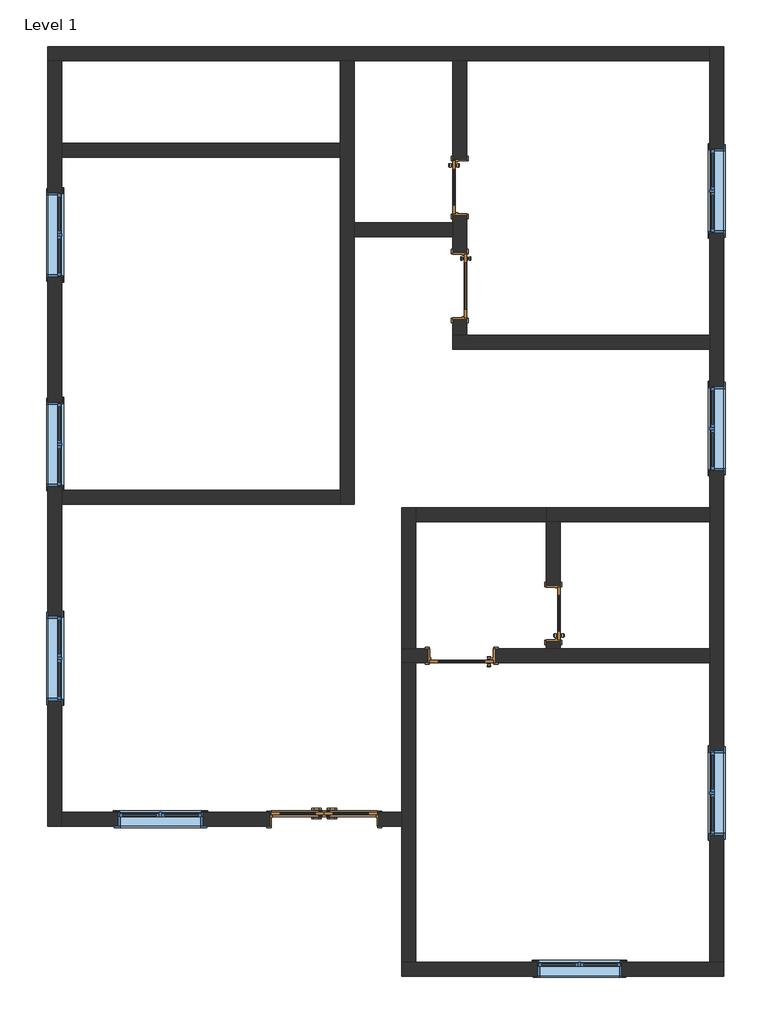
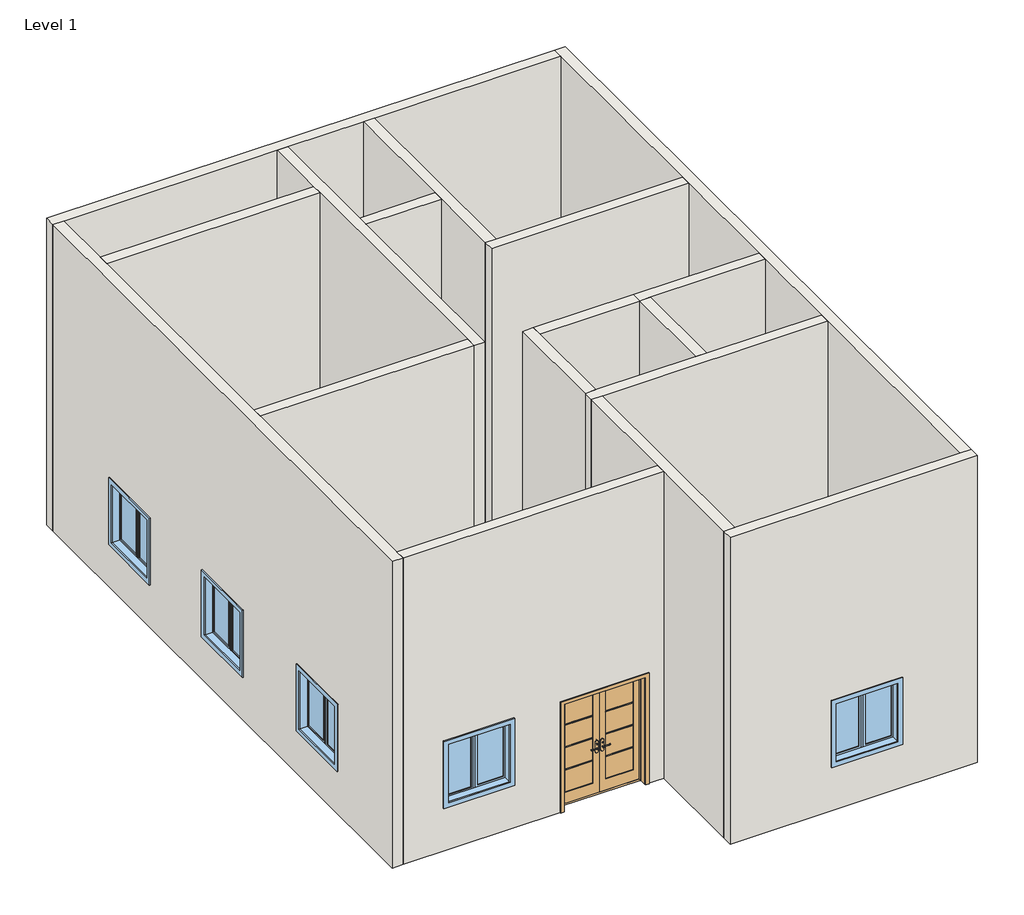
# One storey: 17 walls, 8 windows, 5 doors.
"""IFC4 building model written with IfcOpenShell, lengths in millimetres."""

from ifc_helpers import new_model, si_unit, frame, origin, origin_with_axes, place, context, project, spatial, polyline, outline, extrude, faceted_brep, transform, mapped, element, save
from components import door_34824ff4, door_975671f7, door_b5100634, window_0862ab64

model = new_model("IFC4")

# Units and contexts
model_context = context("Model", 3, world=origin())
ifc_project = project(units=[si_unit("LENGTHUNIT", "METRE", prefix="MILLI")], contexts=[model_context])

# Site, building, storey
site = spatial("IfcSite", under=ifc_project)
building = spatial("IfcBuilding", under=site)
storey = spatial("IfcBuildingStorey", under=building, Name="Level 1", Elevation=0.0)

# Doors
placement = place(None, origin())
door_shape = door_34824ff4(model_context)
element("IfcDoor", 1, ObjectType="Door-Exterior-Double-Full Glass-Wood_Clad : 60\" x 84\"", at=placement, inside=storey, context=model_context, shape_type="MappedRepresentation", body=[
    mapped(door_shape, transform((20054.3621321, 6414.9686058, 0.0), x_axis=(1.0, 0.0, 0.0), y_axis=(0.0, 1.0, 0.0), z_axis=(0.0, 0.0, 1.0))),
])
door_2_shape = door_975671f7(model_context)
element("IfcDoor", 2, ObjectType="Door-Interior-Single-1_Panel-Wood : 30\" x 80\"", at=placement, inside=storey, context=model_context, shape_type="MappedRepresentation", body=[
    mapped(door_2_shape, transform((22006.9871321, 15530.3936058, 0.0), x_axis=(0.0, -1.0, 0.0), y_axis=(1.0, 0.0, 0.0), z_axis=(0.0, 0.0, 1.0))),
])
element("IfcDoor", 3, ObjectType="Door-Interior-Single-1_Panel-Wood : 30\" x 80\"", at=placement, inside=storey, context=model_context, shape_type="MappedRepresentation", body=[
    mapped(door_2_shape, transform((23359.5371321, 9383.5936058, 0.0), x_axis=(0.0, 1.0, 0.0), y_axis=(-1.0, 0.0, 0.0), z_axis=(0.0, 0.0, 1.0))),
])
door_3_shape = door_b5100634(model_context)
element("IfcDoor", 4, ObjectType="Door-Interior-Single-3_Panel_Vert-Wood : 36\" x 80\"", at=placement, inside=storey, context=model_context, shape_type="MappedRepresentation", body=[
    mapped(door_3_shape, transform((22013.3371321, 14107.9936058, 0.0), x_axis=(0.0, -1.0, 0.0), y_axis=(1.0, 0.0, 0.0), z_axis=(0.0, 0.0, 1.0))),
])
element("IfcDoor", 5, ObjectType="Door-Interior-Single-3_Panel_Vert-Wood : 36\" x 80\"", at=placement, inside=storey, context=model_context, shape_type="MappedRepresentation", body=[
    mapped(door_3_shape, transform((22035.5621321, 8770.8186058, 0.0), x_axis=(-1.0, 0.0, 0.0), y_axis=(0.0, -1.0, 0.0), z_axis=(0.0, 0.0, 1.0))),
])

# Walls
element("IfcWall", 6, ObjectType="Generic - 8\"", at=placement, inside=storey, context=model_context, shape_type="Brep", body=[
    faceted_brep([(16066.5621321, 17359.1936058, 0.0), (16269.7621321, 17359.1936058, 0.0), (20282.9621321, 17359.1936058, 0.0), (20486.1621321, 17359.1936058, 0.0), (21908.5621321, 17359.1936058, 0.0), (22111.7621321, 17359.1936058, 0.0), (25616.9621321, 17359.1936058, 0.0), (25616.9621321, 17359.1936058, 6096.0), (22111.7621321, 17359.1936058, 6096.0), (21908.5621321, 17359.1936058, 6096.0), (20486.1621321, 17359.1936058, 6096.0), (20282.9621321, 17359.1936058, 6096.0), (16269.7621321, 17359.1936058, 6096.0), (16066.5621321, 17359.1936058, 6096.0), (16066.5621321, 17562.3936058, 0.0), (16066.5621321, 17562.3936058, 6096.0), (25616.9621321, 17562.3936058, 6096.0), (25616.9621321, 17562.3936058, 0.0)], [[[0, 1, 2, 3, 4, 5, 6, 7, 8, 9, 10, 11, 12, 13]], [[14, 15, 16, 17]], [[6, 5, 4, 3, 2, 1, 0, 14, 17]], [[13, 12, 11, 10, 9, 8, 7, 16, 15]], [[0, 13, 15, 14]], [[7, 6, 17, 16]]]),
])
element("IfcWall", 7, ObjectType="Generic - 8\"", at=placement, inside=storey, context=model_context, shape_type="Brep", body=[
    faceted_brep([(16269.7621321, 6310.1936058, 0.0), (16269.7621321, 6513.3936058, 0.0), (16269.7621321, 10958.3936058, 0.0), (16269.7621321, 11161.5936058, 0.0), (16269.7621321, 15962.1936058, 0.0), (16269.7621321, 16165.3936058, 0.0), (16269.7621321, 17359.1936058, 0.0), (16269.7621321, 17359.1936058, 6096.0), (16269.7621321, 16165.3936058, 6096.0), (16269.7621321, 15962.1936058, 6096.0), (16269.7621321, 11161.5936058, 6096.0), (16269.7621321, 10958.3936058, 6096.0), (16269.7621321, 6513.3936058, 6096.0), (16269.7621321, 6310.1936058, 6096.0), (16269.7621321, 8126.2936058, 2133.6), (16269.7621321, 9345.4936058, 2133.6), (16269.7621321, 9345.4936058, 914.4), (16269.7621321, 8126.2936058, 914.4), (16269.7621321, 11212.3936058, 2133.6), (16269.7621321, 12431.5936058, 2133.6), (16269.7621321, 12431.5936058, 914.4), (16269.7621321, 11212.3936058, 914.4), (16269.7621321, 14234.9936058, 2133.6), (16269.7621321, 15454.1936058, 2133.6), (16269.7621321, 15454.1936058, 914.4), (16269.7621321, 14234.9936058, 914.4), (16066.5621321, 6310.1936058, 0.0), (16066.5621321, 6310.1936058, 6096.0), (16066.5621321, 17359.1936058, 6096.0), (16066.5621321, 17359.1936058, 0.0), (16066.5621321, 8126.2936058, 2133.6), (16066.5621321, 8126.2936058, 914.4), (16066.5621321, 9345.4936058, 914.4), (16066.5621321, 9345.4936058, 2133.6), (16066.5621321, 11212.3936058, 2133.6), (16066.5621321, 11212.3936058, 914.4), (16066.5621321, 12431.5936058, 914.4), (16066.5621321, 12431.5936058, 2133.6), (16066.5621321, 14234.9936058, 2133.6), (16066.5621321, 14234.9936058, 914.4), (16066.5621321, 15454.1936058, 914.4), (16066.5621321, 15454.1936058, 2133.6)], [[[0, 1, 2, 3, 4, 5, 6, 7, 8, 9, 10, 11, 12, 13], [14, 15, 16, 17], [18, 19, 20, 21], [22, 23, 24, 25]], [[26, 27, 28, 29], [30, 31, 32, 33], [34, 35, 36, 37], [38, 39, 40, 41]], [[6, 5, 4, 3, 2, 1, 0, 26, 29]], [[13, 12, 11, 10, 9, 8, 7, 28, 27]], [[7, 6, 29, 28]], [[0, 13, 27, 26]], [[31, 30, 14, 17]], [[32, 31, 17, 16]], [[33, 32, 16, 15]], [[30, 33, 15, 14]], [[35, 34, 18, 21]], [[36, 35, 21, 20]], [[37, 36, 20, 19]], [[34, 37, 19, 18]], [[39, 38, 22, 25]], [[40, 39, 25, 24]], [[41, 40, 24, 23]], [[38, 41, 23, 22]]]),
])
element("IfcWall", 8, ObjectType="Generic - 8\"", at=placement, inside=storey, context=model_context, shape_type="Brep", body=[
    faceted_brep([(25820.1621321, 4354.3936058, 0.0), (25616.9621321, 4354.3936058, 0.0), (21375.1621321, 4354.3936058, 0.0), (21171.9621321, 4354.3936058, 0.0), (21171.9621321, 4354.3936058, 6096.0), (21375.1621321, 4354.3936058, 6096.0), (25616.9621321, 4354.3936058, 6096.0), (25820.1621321, 4354.3936058, 6096.0), (24346.9621321, 4354.3936058, 2133.6), (23127.7621321, 4354.3936058, 2133.6), (23127.7621321, 4354.3936058, 914.4), (24346.9621321, 4354.3936058, 914.4), (25820.1621321, 4151.1936058, 0.0), (25820.1621321, 4151.1936058, 6096.0), (21171.9621321, 4151.1936058, 6096.0), (21171.9621321, 4151.1936058, 0.0), (24346.9621321, 4151.1936058, 2133.6), (24346.9621321, 4151.1936058, 914.4), (23127.7621321, 4151.1936058, 914.4), (23127.7621321, 4151.1936058, 2133.6)], [[[0, 1, 2, 3, 4, 5, 6, 7], [8, 9, 10, 11]], [[12, 13, 14, 15], [16, 17, 18, 19]], [[3, 2, 1, 0, 12, 15]], [[7, 6, 5, 4, 14, 13]], [[0, 7, 13, 12]], [[4, 3, 15, 14]], [[17, 16, 8, 11]], [[18, 17, 11, 10]], [[19, 18, 10, 9]], [[16, 19, 9, 8]]]),
])
element("IfcWall", 9, ObjectType="Generic - 8\"", at=placement, inside=storey, context=model_context, shape_type="Brep", body=[
    faceted_brep([(25616.9621321, 17562.3936058, 0.0), (25616.9621321, 17359.1936058, 0.0), (25616.9621321, 13396.7936058, 0.0), (25616.9621321, 13193.5936058, 0.0), (25616.9621321, 10907.5936058, 0.0), (25616.9621321, 10704.3936058, 0.0), (25616.9621321, 8875.5936058, 0.0), (25616.9621321, 8672.3936058, 0.0), (25616.9621321, 4354.3936058, 0.0), (25616.9621321, 4354.3936058, 6096.0), (25616.9621321, 8672.3936058, 6096.0), (25616.9621321, 8875.5936058, 6096.0), (25616.9621321, 10704.3936058, 6096.0), (25616.9621321, 10907.5936058, 6096.0), (25616.9621321, 13193.5936058, 6096.0), (25616.9621321, 13396.7936058, 6096.0), (25616.9621321, 17359.1936058, 6096.0), (25616.9621321, 17562.3936058, 6096.0), (25616.9621321, 7402.3936058, 2133.6), (25616.9621321, 6183.1936058, 2133.6), (25616.9621321, 6183.1936058, 914.4), (25616.9621321, 7402.3936058, 914.4), (25616.9621321, 12660.1936058, 2133.6), (25616.9621321, 11440.9936058, 2133.6), (25616.9621321, 11440.9936058, 914.4), (25616.9621321, 12660.1936058, 914.4), (25616.9621321, 16089.1936058, 2133.6), (25616.9621321, 14869.9936058, 2133.6), (25616.9621321, 14869.9936058, 914.4), (25616.9621321, 16089.1936058, 914.4), (25820.1621321, 17562.3936058, 0.0), (25820.1621321, 17562.3936058, 6096.0), (25820.1621321, 4354.3936058, 6096.0), (25820.1621321, 4354.3936058, 0.0), (25820.1621321, 7402.3936058, 2133.6), (25820.1621321, 7402.3936058, 914.4), (25820.1621321, 6183.1936058, 914.4), (25820.1621321, 6183.1936058, 2133.6), (25820.1621321, 12660.1936058, 2133.6), (25820.1621321, 12660.1936058, 914.4), (25820.1621321, 11440.9936058, 914.4), (25820.1621321, 11440.9936058, 2133.6), (25820.1621321, 16089.1936058, 2133.6), (25820.1621321, 16089.1936058, 914.4), (25820.1621321, 14869.9936058, 914.4), (25820.1621321, 14869.9936058, 2133.6)], [[[0, 1, 2, 3, 4, 5, 6, 7, 8, 9, 10, 11, 12, 13, 14, 15, 16, 17], [18, 19, 20, 21], [22, 23, 24, 25], [26, 27, 28, 29]], [[30, 31, 32, 33], [34, 35, 36, 37], [38, 39, 40, 41], [42, 43, 44, 45]], [[8, 7, 6, 5, 4, 3, 2, 1, 0, 30, 33]], [[17, 16, 15, 14, 13, 12, 11, 10, 9, 32, 31]], [[0, 17, 31, 30]], [[9, 8, 33, 32]], [[35, 34, 18, 21]], [[36, 35, 21, 20]], [[37, 36, 20, 19]], [[34, 37, 19, 18]], [[39, 38, 22, 25]], [[40, 39, 25, 24]], [[41, 40, 24, 23]], [[38, 41, 23, 22]], [[43, 42, 26, 29]], [[44, 43, 29, 28]], [[45, 44, 28, 27]], [[42, 45, 27, 26]]]),
])
element("IfcWall", 10, ObjectType="Generic - 8\"", at=placement, inside=storey, context=model_context, shape_type="Brep", body=[
    faceted_brep([(25616.9621321, 13396.7936058, 0.0), (22111.7621321, 13396.7936058, 0.0), (21908.5621321, 13396.7936058, 0.0), (21908.5621321, 13396.7936058, 6096.0), (22111.7621321, 13396.7936058, 6096.0), (25616.9621321, 13396.7936058, 6096.0), (25616.9621321, 13193.5936058, 0.0), (25616.9621321, 13193.5936058, 6096.0), (21908.5621321, 13193.5936058, 6096.0), (21908.5621321, 13193.5936058, 0.0)], [[[0, 1, 2, 3, 4, 5]], [[6, 7, 8, 9]], [[2, 1, 0, 6, 9]], [[3, 2, 9, 8]], [[5, 4, 3, 8, 7]], [[0, 5, 7, 6]]]),
])
element("IfcWall", 11, ObjectType="Generic - 8\"", at=placement, inside=storey, context=model_context, shape_type="Brep", body=[
    faceted_brep([(22111.7621321, 17359.1936058, 6096.0), (22111.7621321, 13396.7936058, 6096.0), (22111.7621321, 13396.7936058, 0.0), (22111.7621321, 13625.3936058, 0.0), (22111.7621321, 13625.3936058, 2057.4), (22111.7621321, 14590.5936058, 2057.4), (22111.7621321, 14590.5936058, 0.0), (22111.7621321, 15123.9936058, 0.0), (22111.7621321, 15123.9936058, 2057.4), (22111.7621321, 15936.7936058, 2057.4), (22111.7621321, 15936.7936058, 0.0), (22111.7621321, 17359.1936058, 0.0), (21908.5621321, 13396.7936058, 6096.0), (21908.5621321, 14819.1936058, 6096.0), (21908.5621321, 15022.3936058, 6096.0), (21908.5621321, 17359.1936058, 6096.0), (21908.5621321, 17359.1936058, 0.0), (21908.5621321, 15936.7936058, 0.0), (21908.5621321, 15936.7936058, 2057.4), (21908.5621321, 15123.9936058, 2057.4), (21908.5621321, 15123.9936058, 0.0), (21908.5621321, 15022.3936058, 0.0), (21908.5621321, 14819.1936058, 0.0), (21908.5621321, 14590.5936058, 0.0), (21908.5621321, 14590.5936058, 2057.4), (21908.5621321, 13625.3936058, 2057.4), (21908.5621321, 13625.3936058, 0.0), (21908.5621321, 13396.7936058, 0.0)], [[[0, 1, 2, 3, 4, 5, 6, 7, 8, 9, 10, 11]], [[12, 13, 14, 15, 16, 17, 18, 19, 20, 21, 22, 23, 24, 25, 26, 27]], [[2, 27, 26, 3]], [[16, 11, 10, 17]], [[6, 23, 22, 21, 20, 7]], [[1, 0, 15, 14, 13, 12]], [[0, 11, 16, 15]], [[2, 1, 12, 27]], [[25, 4, 3, 26]], [[4, 25, 24, 5]], [[5, 24, 23, 6]], [[19, 8, 7, 20]], [[8, 19, 18, 9]], [[9, 18, 17, 10]]]),
])
element("IfcWall", 12, ObjectType="Generic - 8\"", at=placement, inside=storey, context=model_context, shape_type="SweptSolid", body=[
    extrude(outline(polyline([(20486.1621321, 15022.3936058), (21908.5621321, 15022.3936058), (21908.5621321, 14819.1936058), (20486.1621321, 14819.1936058), (20486.1621321, 15022.3936058)])), origin_with_axes(), (0.0, 0.0, 1.0), 6096.0),
])
element("IfcWall", 13, ObjectType="Generic - 8\"", at=placement, inside=storey, context=model_context, shape_type="Brep", body=[
    faceted_brep([(20486.1621321, 10958.3936058, 0.0), (20486.1621321, 14819.1936058, 0.0), (20486.1621321, 15022.3936058, 0.0), (20486.1621321, 17359.1936058, 0.0), (20486.1621321, 17359.1936058, 6096.0), (20486.1621321, 15022.3936058, 6096.0), (20486.1621321, 14819.1936058, 6096.0), (20486.1621321, 10958.3936058, 6096.0), (20282.9621321, 10958.3936058, 0.0), (20282.9621321, 10958.3936058, 6096.0), (20282.9621321, 11161.5936058, 6096.0), (20282.9621321, 15962.1936058, 6096.0), (20282.9621321, 16165.3936058, 6096.0), (20282.9621321, 17359.1936058, 6096.0), (20282.9621321, 17359.1936058, 0.0), (20282.9621321, 16165.3936058, 0.0), (20282.9621321, 15962.1936058, 0.0), (20282.9621321, 11161.5936058, 0.0)], [[[0, 1, 2, 3, 4, 5, 6, 7]], [[8, 9, 10, 11, 12, 13, 14, 15, 16, 17]], [[3, 2, 1, 0, 8, 17, 16, 15, 14]], [[7, 6, 5, 4, 13, 12, 11, 10, 9]], [[4, 3, 14, 13]], [[0, 7, 9, 8]]]),
])
element("IfcWall", 14, ObjectType="Generic - 8\"", at=placement, inside=storey, context=model_context, shape_type="SweptSolid", body=[
    extrude(outline(polyline([(16269.7621321, 16165.3936058), (20282.9621321, 16165.3936058), (20282.9621321, 15962.1936058), (16269.7621321, 15962.1936058), (16269.7621321, 16165.3936058)])), origin_with_axes(), (0.0, 0.0, 1.0), 6096.0),
])
element("IfcWall", 15, ObjectType="Generic - 8\"", at=placement, inside=storey, context=model_context, shape_type="SweptSolid", body=[
    extrude(outline(polyline([(20282.9621321, 10958.3936058), (16269.7621321, 10958.3936058), (16269.7621321, 11161.5936058), (20282.9621321, 11161.5936058), (20282.9621321, 10958.3936058)])), origin_with_axes(), (0.0, 0.0, 1.0), 6096.0),
])
element("IfcWall", 16, ObjectType="Generic - 8\"", at=placement, inside=storey, context=model_context, shape_type="Brep", body=[
    faceted_brep([(21171.9621321, 8875.5936058, 6096.0), (21375.1621321, 8875.5936058, 6096.0), (23254.7621321, 8875.5936058, 6096.0), (23457.9621321, 8875.5936058, 6096.0), (25616.9621321, 8875.5936058, 6096.0), (25616.9621321, 8875.5936058, 0.0), (23457.9621321, 8875.5936058, 0.0), (23254.7621321, 8875.5936058, 0.0), (22518.1621321, 8875.5936058, 0.0), (22518.1621321, 8875.5936058, 2057.4), (21552.9621321, 8875.5936058, 2057.4), (21552.9621321, 8875.5936058, 0.0), (21375.1621321, 8875.5936058, 0.0), (21171.9621321, 8875.5936058, 0.0), (25616.9621321, 8672.3936058, 6096.0), (21375.1621321, 8672.3936058, 6096.0), (21171.9621321, 8672.3936058, 6096.0), (21171.9621321, 8672.3936058, 0.0), (21375.1621321, 8672.3936058, 0.0), (21552.9621321, 8672.3936058, 0.0), (21552.9621321, 8672.3936058, 2057.4), (22518.1621321, 8672.3936058, 2057.4), (22518.1621321, 8672.3936058, 0.0), (25616.9621321, 8672.3936058, 0.0)], [[[0, 1, 2, 3, 4, 5, 6, 7, 8, 9, 10, 11, 12, 13]], [[14, 15, 16, 17, 18, 19, 20, 21, 22, 23]], [[5, 23, 22, 8, 7, 6]], [[17, 13, 12, 11, 19, 18]], [[4, 3, 2, 1, 0, 16, 15, 14]], [[5, 4, 14, 23]], [[0, 13, 17, 16]], [[10, 20, 19, 11]], [[20, 10, 9, 21]], [[21, 9, 8, 22]]]),
])
element("IfcWall", 17, ObjectType="Generic - 8\"", at=placement, inside=storey, context=model_context, shape_type="Brep", body=[
    faceted_brep([(21171.9621321, 8672.3936058, 0.0), (21171.9621321, 6513.3936058, 0.0), (21171.9621321, 6310.1936058, 0.0), (21171.9621321, 4354.3936058, 0.0), (21171.9621321, 4354.3936058, 6096.0), (21171.9621321, 6310.1936058, 6096.0), (21171.9621321, 6513.3936058, 6096.0), (21171.9621321, 8672.3936058, 6096.0), (21375.1621321, 8672.3936058, 0.0), (21375.1621321, 8672.3936058, 6096.0), (21375.1621321, 4354.3936058, 6096.0), (21375.1621321, 4354.3936058, 0.0)], [[[0, 1, 2, 3, 4, 5, 6, 7]], [[8, 9, 10, 11]], [[3, 2, 1, 0, 8, 11]], [[7, 6, 5, 4, 10, 9]], [[0, 7, 9, 8]], [[4, 3, 11, 10]]]),
])
element("IfcWall", 18, ObjectType="Generic - 8\"", at=placement, inside=storey, context=model_context, shape_type="Brep", body=[
    faceted_brep([(25616.9621321, 10907.5936058, 0.0), (23254.7621321, 10907.5936058, 0.0), (23254.7621321, 10907.5936058, 6096.0), (25616.9621321, 10907.5936058, 6096.0), (25616.9621321, 10704.3936058, 0.0), (25616.9621321, 10704.3936058, 6096.0), (23457.9621321, 10704.3936058, 6096.0), (23254.7621321, 10704.3936058, 6096.0), (23254.7621321, 10704.3936058, 0.0), (23457.9621321, 10704.3936058, 0.0)], [[[0, 1, 2, 3]], [[4, 5, 6, 7, 8, 9]], [[1, 0, 4, 9, 8]], [[3, 2, 7, 6, 5]], [[0, 3, 5, 4]], [[2, 1, 8, 7]]]),
])
element("IfcWall", 19, ObjectType="Generic - 8\"", at=placement, inside=storey, context=model_context, shape_type="SweptSolid", body=[
    extrude(outline(polyline([(8875.5936058, 6096.0), (10704.3936058, 6096.0), (10704.3936058, 0.0), (9789.9936058, 0.0), (9789.9936058, 2057.4), (8977.1936058, 2057.4), (8977.1936058, 0.0), (8875.5936058, 0.0), (8875.5936058, 6096.0)])), frame((23254.7621321, 0.0, 0.0), z_axis=(1.0, 0.0, 0.0), x_axis=(0.0, 1.0, 0.0)), (0.0, 0.0, 1.0), 203.2),
])
element("IfcWall", 20, ObjectType="Generic - 8\"", at=placement, inside=storey, context=model_context, shape_type="Brep", body=[
    faceted_brep([(21375.1621321, 8875.5936058, 0.0), (21375.1621321, 10704.3936058, 0.0), (21375.1621321, 10907.5936058, 0.0), (21375.1621321, 10907.5936058, 6096.0), (21375.1621321, 10704.3936058, 6096.0), (21375.1621321, 8875.5936058, 6096.0), (21171.9621321, 8875.5936058, 0.0), (21171.9621321, 8875.5936058, 6096.0), (21171.9621321, 10907.5936058, 6096.0), (21171.9621321, 10907.5936058, 0.0)], [[[0, 1, 2, 3, 4, 5]], [[6, 7, 8, 9]], [[2, 1, 0, 6, 9]], [[5, 4, 3, 8, 7]], [[0, 5, 7, 6]], [[3, 2, 9, 8]]]),
])
element("IfcWall", 21, ObjectType="Generic - 8\"", at=placement, inside=storey, context=model_context, shape_type="SweptSolid", body=[
    extrude(outline(polyline([(21375.1621321, 10907.5936058), (23254.7621321, 10907.5936058), (23254.7621321, 10704.3936058), (21375.1621321, 10704.3936058), (21375.1621321, 10907.5936058)])), origin_with_axes(), (0.0, 0.0, 1.0), 6096.0),
])
element("IfcWall", 22, ObjectType="Generic - 8\"", at=placement, inside=storey, context=model_context, shape_type="SweptSolid", body=[
    extrude(outline(polyline([(6096.0, 21171.9621321), (6096.0, 16269.7621321), (0.0, 16269.7621321), (0.0, 19266.9621321), (2159.0, 19266.9621321), (2159.0, 20841.7621321), (0.0, 20841.7621321), (0.0, 21171.9621321), (6096.0, 21171.9621321)]), holes=[polyline([(2133.6, 18301.7621321), (914.4, 18301.7621321), (914.4, 17082.5621321), (2133.6, 17082.5621321), (2133.6, 18301.7621321)])]), frame((0.0, 6310.1936058, 0.0), z_axis=(0.0, 1.0, 0.0), x_axis=(0.0, 0.0, 1.0)), (0.0, 0.0, 1.0), 203.2),
])

# Windows
window_shape = window_0862ab64(model_context)
element("IfcWindow", 23, ObjectType="Casement Dbl with Trim : 48\" x 48\"", at=placement, inside=storey, context=model_context, shape_type="MappedRepresentation", body=[
    mapped(window_shape, transform((16149.1121321, 8735.8936058, 0.0), x_axis=(0.0, -1.0, 0.0), y_axis=(1.0, 0.0, 0.0), z_axis=(0.0, 0.0, 1.0))),
])
element("IfcWindow", 24, ObjectType="Casement Dbl with Trim : 48\" x 48\"", at=placement, inside=storey, context=model_context, shape_type="MappedRepresentation", body=[
    mapped(window_shape, transform((16149.1121321, 11821.9936058, 0.0), x_axis=(0.0, -1.0, 0.0), y_axis=(1.0, 0.0, 0.0), z_axis=(0.0, 0.0, 1.0))),
])
element("IfcWindow", 25, ObjectType="Casement Dbl with Trim : 48\" x 48\"", at=placement, inside=storey, context=model_context, shape_type="MappedRepresentation", body=[
    mapped(window_shape, transform((16149.1121321, 14844.5936058, 0.0), x_axis=(0.0, -1.0, 0.0), y_axis=(1.0, 0.0, 0.0), z_axis=(0.0, 0.0, 1.0))),
])
element("IfcWindow", 26, ObjectType="Casement Dbl with Trim : 48\" x 48\"", at=placement, inside=storey, context=model_context, shape_type="MappedRepresentation", body=[
    mapped(window_shape, transform((17692.1621321, 6392.7436058, 0.0), x_axis=(1.0, 0.0, 0.0), y_axis=(0.0, 1.0, 0.0), z_axis=(0.0, 0.0, 1.0))),
])
element("IfcWindow", 27, ObjectType="Casement Dbl with Trim : 48\" x 48\"", at=placement, inside=storey, context=model_context, shape_type="MappedRepresentation", body=[
    mapped(window_shape, transform((23737.3621321, 4233.7436058, 0.0), x_axis=(1.0, 0.0, 0.0), y_axis=(0.0, 1.0, 0.0), z_axis=(0.0, 0.0, 1.0))),
])
element("IfcWindow", 28, ObjectType="Casement Dbl with Trim : 48\" x 48\"", at=placement, inside=storey, context=model_context, shape_type="MappedRepresentation", body=[
    mapped(window_shape, transform((25737.6121321, 6792.7936058, 0.0), x_axis=(0.0, 1.0, 0.0), y_axis=(-1.0, 0.0, 0.0), z_axis=(0.0, 0.0, 1.0))),
])
element("IfcWindow", 29, ObjectType="Casement Dbl with Trim : 48\" x 48\"", at=placement, inside=storey, context=model_context, shape_type="MappedRepresentation", body=[
    mapped(window_shape, transform((25737.6121321, 12050.5936058, 0.0), x_axis=(0.0, 1.0, 0.0), y_axis=(-1.0, 0.0, 0.0), z_axis=(0.0, 0.0, 1.0))),
])
element("IfcWindow", 30, ObjectType="Casement Dbl with Trim : 48\" x 48\"", at=placement, inside=storey, context=model_context, shape_type="MappedRepresentation", body=[
    mapped(window_shape, transform((25737.6121321, 15479.5936058, 0.0), x_axis=(0.0, 1.0, 0.0), y_axis=(-1.0, 0.0, 0.0), z_axis=(0.0, 0.0, 1.0))),
])

save(model, "model.ifc")

# Revit data of these elements
# Type "Door-Exterior-Double-Full Glass-Wood_Clad : 60\" x 84\""
#   Type Mark = "8"
#   Assembly Code = "B2030100"
#   Analytic Construction = "French door, wood frame with double glass"
#   Top Rail = 0' - 4 11/16"
#   Threshold Offset [instance default] = 0' - 0 1/2"
#   Thickness = 0' - 1 3/8"
#   Thermal Resistance (R) = 0.337392 (m²·K)/W
#   Swing Angle [instance default] = 90.00°
#   Stiles = 0' - 4 3/4"
#   Rough Width = 5' - 2"
#   Rough Height = 7' - 1"
#   Panel Width = 2' - 6"
#   Door Offset [instance default] = 0' - 0"
#   Height = 7' - 0"
#   Width = 5' - 0"
#   Heat Transfer Coefficient (U) = 2.96405 W/(m²·K)
#   Bottom Rail = 0' - 9 1/8"
#   Exterior Trim [instance default] = yes
#   Threshold [instance default] = yes
#   Show Grill [instance default] = yes
#   Function = 1
#   Trim Material = Cherry
#   Threshold Material = Cherry
#   Panel Material = Cherry
#   Glazing = Glass
#   Frame Material = Cherry
#   Door Handle Material = Aluminum
#   Visual Light Transmittance = 0
#   Solar Heat Gain Coefficient = 0
#   Wall Closure = (empty or 0)
#   Construction Type = (empty or 0)
# Type "Door-Interior-Single-1_Panel-Wood : 30\" x 80\""
#   Type Mark = "10"
#   Assembly Code = "C1020300"
#   Analytic Construction = "Wooden"
#   Top Rail = 0' - 4 11/16"
#   Thickness = 0' - 1 3/8"
#   Thermal Resistance (R) = 0.455703 (m²·K)/W
#   Swing Angle [instance default] = 90.00°
#   Stiles = 0' - 4 3/4"
#   Rough Width = 2' - 8"
#   Rough Height = 6' - 9"
#   Height = 6' - 8"
#   Width = 2' - 6"
#   Heat Transfer Coefficient (U) = 2.19465 W/(m²·K)
#   Bottom Rail = 0' - 9 1/8"
#   Trim Material = Cherry
#   Panel Material = Cherry
#   Frame Material = Cherry
#   Door Handle Material = Aluminum
#   Visual Light Transmittance = 0
#   Solar Heat Gain Coefficient = 0
#   Wall Closure = (empty or 0)
#   Function = (empty or 0)
# Type "Door-Interior-Single-3_Panel_Vert-Wood : 36\" x 80\""
#   Type Mark = "9"
#   Assembly Code = "C1020300"
#   Analytic Construction = "Wooden"
#   Top Rail = 0' - 4 11/16"
#   Thickness = 0' - 1 3/8"
#   Thermal Resistance (R) = 0.455703 (m²·K)/W
#   Swing Angle [instance default] = 90.00°
#   Stiles = 0' - 4 3/4"
#   Rough Width = 3' - 2"
#   Rough Height = 6' - 9"
#   Intermediate Rail = 0' - 4 1/2"
#   Height = 6' - 8"
#   Width = 3' - 0"
#   Heat Transfer Coefficient (U) = 2.19465 W/(m²·K)
#   Bottom Rail = 0' - 9 1/8"
#   Trim Material = Cherry
#   Panel Material = Cherry
#   Frame Material = Cherry
#   Door Handle Material = Aluminum
#   Visual Light Transmittance = 0
#   Solar Heat Gain Coefficient = 0
#   Wall Closure = (empty or 0)
#   Function = (empty or 0)
# Type "Generic - 8\""
#   Assembly Code = "B2010"
#   Width = 0' - 8"
#   Layers, outside or top first: 0' - 8" no material (function 1)
# Type "Casement Dbl with Trim : 48\" x 48\""
#   Type Mark = "10"
#   Construction Type Id = "GSP4R"
#   Assembly Code = "B2020100"
#   Analytic Construction = "1/8 in Pilkington single glazing"
#   Visual Light Transmittance = 0.9
#   Solar Heat Gain Coefficient = 0.78
#   Heat Transfer Coefficient (U) = 3.6886 W/(m²·K)
#   Height = 4' - 0"
#   Default Sill Height = 3' - 0"
#   Trim Projection - Ext. = 0' - 0 1/2"
#   Trim Projection - Int. = 0' - 0 3/4"
#   Trim Width - Exterior = 0' - 3 1/2"
#   Trim Width - Interior = 0' - 3 1/2"
#   Width = 4' - 0"
#   Window Inset = 0' - 0 3/4"
#   Glass Pane Material = Glass
#   Sash Material = Sash
#   Trim Exterior Material = Trim
#   Trim Interior Material = Trim
#   Wall Closure = (empty or 0)
# Element 1 (IfcDoor, "Door-Exterior-Double-Full Glass-Wood_Clad : 60\" x 84\"")
#   Threshold Offset = 0' - 0 1/2"
#   Swing Angle = 90.00°
#   Door Offset = 0' - 0"
#   Threshold = yes
#   Show Grill = yes
#   Exterior Trim = yes
#   Phase Created = New Construction
#   Materials on its faces: "Cherry", "Aluminum", "Glass"
# Elements 2, 3 (IfcDoor, "Door-Interior-Single-1_Panel-Wood : 30\" x 80\"")
#   Swing Angle = 90.00°
#   Phase Created = New Construction
#   Materials on its faces: "Cherry", "Aluminum"
# Elements 4, 5 (IfcDoor, "Door-Interior-Single-3_Panel_Vert-Wood : 36\" x 80\"")
#   Swing Angle = 90.00°
#   Phase Created = New Construction
#   Materials on its faces: "Cherry", "Aluminum"
# Elements 6, 7, 8, 9, 10, 11, 12, 13, 14, 15, 16, 17, 18, 19, 20, 21, 22 (IfcWall, "Generic - 8\"")
#   Top Offset = 0' - 0"
#   Base Offset = 0' - 0"
#   Unconnected Height = 20' - 0"
#   wall height = 20' - 0"
#   Phase Created = New Construction
#   Base Constraint = Level 1
#   Materials on its faces: "Default Wall"
# Element 23 (IfcWindow, "Casement Dbl with Trim : 48\" x 48\"")
#   Mark = "1"
#   Phase Created = New Construction
#   Materials on its faces: "Sash", "Trim", "Glass"
# Element 24 (IfcWindow, "Casement Dbl with Trim : 48\" x 48\"")
#   Mark = "2"
#   Phase Created = New Construction
#   Materials on its faces: "Sash", "Trim", "Glass"
# Element 25 (IfcWindow, "Casement Dbl with Trim : 48\" x 48\"")
#   Mark = "3"
#   Phase Created = New Construction
#   Materials on its faces: "Sash", "Trim", "Glass"
# Element 26 (IfcWindow, "Casement Dbl with Trim : 48\" x 48\"")
#   Mark = "4"
#   Phase Created = New Construction
#   Materials on its faces: "Sash", "Trim", "Glass"
# Element 27 (IfcWindow, "Casement Dbl with Trim : 48\" x 48\"")
#   Mark = "5"
#   Phase Created = New Construction
#   Materials on its faces: "Sash", "Trim", "Glass"
# Element 28 (IfcWindow, "Casement Dbl with Trim : 48\" x 48\"")
#   Mark = "6"
#   Phase Created = New Construction
#   Materials on its faces: "Sash", "Trim", "Glass"
# Element 29 (IfcWindow, "Casement Dbl with Trim : 48\" x 48\"")
#   Mark = "7"
#   Phase Created = New Construction
#   Materials on its faces: "Sash", "Trim", "Glass"
# Element 30 (IfcWindow, "Casement Dbl with Trim : 48\" x 48\"")
#   Mark = "8"
#   Phase Created = New Construction
#   Materials on its faces: "Sash", "Trim", "Glass"
# Materials
#   "Cherry": class "Wood", colour RGB 226 177 128, transparency 0, Description = "Prunus Serotina", Cost = 0
#   "Glass": class "Glass", colour RGB 0 128 192, transparency 0.75, Description = "Soda Lime Glass", Cost = 0
#   "Aluminum": class "Metal", colour RGB 247 247 247, transparency 0, Description = "Aluminum 6061", Cost = 0
#   "Sash": class "Wood", colour RGB 224 178 126, transparency 0
#   "Trim": class "Wood", colour RGB 224 178 126, transparency 0
#   "Default Wall": colour RGB 128 128 128, transparency 0
